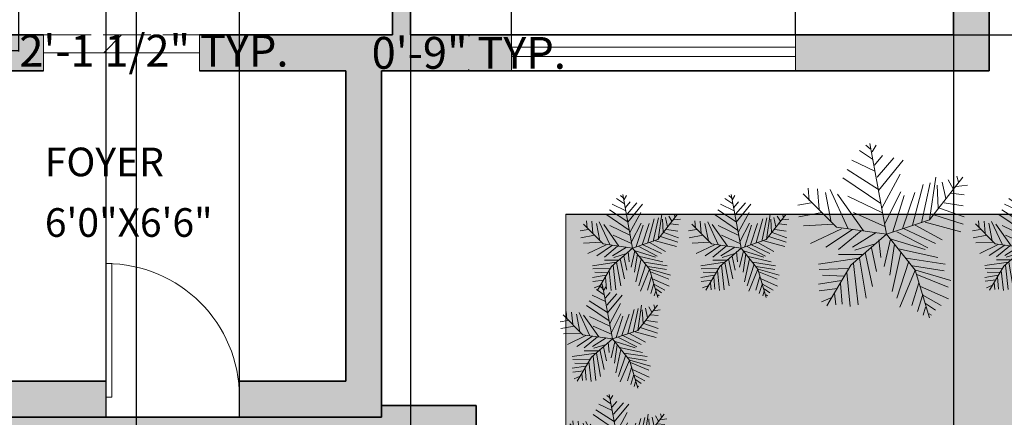
# Model space of a CAD drawing. Units: inches. Extents: x 853 to 1550, y 485 to 1596.
# Tile 5 of 18: x 1170 to 1418, y 768 to 867. Entities that reach past the tile are written whole.
import ezdxf

# ---------------------------------------------------------------- set-up
doc = ezdxf.new("R2010")
doc.units = ezdxf.units.IN
doc.header["$MEASUREMENT"] = 0
doc.linetypes.add('ACAD_ISO02W100', pattern=[15, 12, -3])
for name, color, linetype, lineweight in [('A-ANNO-DIMS', 2, 'Continuous', 18), ('A-AREA-IDEN', 250, 'Continuous', 18), ('A-DOOR', 4, 'Continuous', 18), ('A-GLAZ-HIDN', 4, 'ACAD_ISO02W100', 13), ('A-WALL-PATT', 250, 'Continuous', 13), ('L-PLNT-TREE', 106, 'Continuous', 13), ('lawn', 106, 'Continuous', 18), ('walls', 250, 'Continuous', 35), ('windows', 4, 'Continuous', 18)]:
    doc.layers.add(name, color=color, linetype=linetype, lineweight=lineweight)
doc.layers.add('A-FLOR-PATT', color=254, linetype='Continuous', lineweight=13, true_color=0xfeeab9)
doc.layers.add('L-PLNT-PATT', color=85, linetype='Continuous', lineweight=13, true_color=0x58ba48)
doc.styles.get("Standard").update_dxf_attribs({"font": 'arial.ttf'})
doc.dimstyles.get("Standard").update_dxf_attribs({"dimtxt": 8, "dimasz": 0.18, "dimexe": 0.18, "dimexo": 0.0625, "dimgap": 0.09, "dimtad": 0, "dimtih": 1, "dimtoh": 1, "dimzin": 0, "dimdsep": 46, "dimlunit": 3, "dimtxsty": 'Standard', "dimcen": 0.09, "dimadec": 0, "dimazin": 0, "dimtfac": 1, "dimtofl": 0, "dimtmove": 0, "dimatfit": 3, "dimfxl": 1, "dimtolj": 1, "dimtzin": 0, "dimarcsym": 0})

# ---------------------------------------------------------------- blocks, each defined once
blk = doc.blocks.new('*U10')
for p, q in [((0, 0), (0, -6)), ((40, 0), (40, -6))]:
    blk.add_line(p, q)
blk.add_lwpolyline([(0, 0), (0, 40), (1.75, 40), (1.75, 0)], close=True)
blk.add_arc((0, 0), 40, 0, 90)
blk = doc.blocks.new('*U18')
for p, q in [((-10.186, 53.64), (-13.084, 55.962)), ((0, 0), (-10.5, 57)), ((-9.099, 51.782), (-6.563, 55.962)), ((-8.737, 47.138), (-17.069, 52.711)), ((-7.288, 39.707), (-21.778, 46.673)), ((-7.65, 43.423), (-2.578, 49.46)), ((-5.839, 35.992), (4.667, 48.067)), ((-5.114, 27.632), (10.463, 46.673)), ((-5.114, 28.097), (-24.676, 40.636)), ((-2.941, 16.486), (8.652, 37.85)), ((-3.665, 19.273), (-27.574, 35.527)), ((16.259, 5.805), (23.142, 31.348)), ((22.055, 7.198), (27.489, 32.277)), ((27, 9), (48, 36)), ((27.127, 9.056), (31.112, 35.992)), ((35.096, 32.741), (37.27, 22.524)), ((38.719, 34.134), (41.979, 28.561)), ((44.153, 36.456), (45.239, 32.741)), ((-31.5, 4.5), (-52.5, 25.5)), ((-48.585, 21.131), (-49.309, 29.026)), ((-43.513, 28.561), (-42.427, 15.558)), ((-38.442, 26.239), (-34.819, 7.663)), ((-35.544, 28.097), (-24.314, 3.947)), ((-14.533, 2.09), (-30.834, 25.31)), ((-1.129, 6.734), (9.014, 26.704)), ((10.101, 3.483), (17.708, 26.239)), ((31.836, 30.883), (32.561, 16.486)), ((40.53, 25.775), (48.862, 24.846)), ((43.791, 29.954), (51.036, 30.883)), ((-47.498, 19.737), (-55.83, 18.344)), ((-24.314, 23.917), (-2.941, 13.7)), ((3.942, 1.625), (11.187, 24.381)), ((36.183, 19.737), (48.137, 17.88)), ((-40.615, 13.7), (-55.105, 10.913)), ((-20.691, 13.7), (-1.129, 4.876)), ((33.285, 16.486), (48.862, 10.913)), ((-33.37, 6.269), (-52.207, 5.34)), ((0, 0), (27, 9)), ((24.229, 7.663), (46.688, 1.625)), ((29.662, 12.307), (48.137, 6.269)), ((-28.299, 3.483), (-47.86, -5.805)), ((-21.416, 3.018), (-38.079, -8.128)), ((0, 0), (-31.5, 4.5)), ((-15.982, 2.09), (-30.11, -9.521)), ((0, 0), (-22.5, -19.5)), ((-6.563, 1.161), (-21.416, -8.128)), ((0, 0), (18, -22.5)), ((6.478, 1.625), (26.04, -8.592)), ((11.187, 3.483), (30.749, -5.805)), ((18.07, 5.805), (35.096, -3.483)), ((-6.563, -5.805), (-19.967, -9.985)), ((-4.752, -3.483), (-3.665, -14.629)), ((2.493, -3.019), (-1.491, -20.202)), ((1.769, -2.555), (24.229, -9.521)), ((-13.446, -11.378), (-8.737, -32.741)), ((-9.461, -8.592), (-6.201, -23.453)), ((5.029, -6.27), (2.131, -25.775)), ((9.014, -11.378), (3.58, -35.992)), ((7.565, -9.056), (32.198, -14.629)), ((-17.431, -15.094), (-42.789, -18.809)), ((-15.257, -12.772), (-30.11, -12.772)), ((-20.691, -18.345), (-17.793, -44.352)), ((-17.069, -15.094), (-12.721, -40.172)), ((14.085, -16.951), (6.478, -40.172)), ((12.274, -15.094), (36.907, -18.809)), ((-24.314, -21.596), (-42.427, -22.06)), ((-22.5, -19.5), (-37.5, -45)), ((-25.038, -23.918), (-22.865, -45.281)), ((18.07, -22.524), (8.289, -45.745)), ((16.259, -19.738), (36.183, -22.989)), ((18, -22.5), (27, -52.5)), ((18.433, -22.524), (40.53, -29.026)), ((-28.299, -29.026), (-42.789, -31.348)), ((-26.849, -26.24), (-40.253, -25.775)), ((-29.023, -30.884), (-27.936, -43.887)), ((20.244, -30.419), (15.897, -44.816)), ((19.157, -25.311), (38.719, -33.206)), ((-30.834, -34.135), (-42.427, -35.528)), ((-32.646, -36.921), (-31.921, -44.352)), ((21.331, -32.741), (39.081, -40.636)), ((-34.457, -39.708), (-40.978, -42.494)), ((22.78, -37.85), (19.519, -48.532)), ((22.78, -38.314), (34.372, -44.816)), ((24.591, -45.745), (23.142, -50.854)), ((24.591, -43.423), (30.749, -47.603)), ((26.764, -49.925), (28.213, -50.854))]:
    blk.add_line(p, q)
blk = doc.blocks.new('WIN-71IN')
for p, q in [((0, 9), (0, 0)), ((71.43, 9), (0, 9)), ((0, 9), (0, 5.92)), ((71.43, 0), (71.43, 9)), ((0, 5.92), (71.43, 5.92)), ((71.43, 5.92), (71.43, 3.59)), ((71.43, 3.59), (0, 3.59)), ((0, 0), (71.43, 0))]:
    blk.add_line(p, q)
blk = doc.blocks.new('*D41')
at = {"layer": 'A-ANNO-DIMS', "color": 0, "lineweight": -2, "transparency": 16777216}
for p, q in [((1293.81, 863.69), (1293.81, 874.52)), ((1293.99, 874.34), (1365.06, 874.34)), ((1365.24, 863.69), (1365.24, 874.52)), ((1365.24, 874.34), (1365.42, 874.34))]:
    blk.add_line(p, q, dxfattribs=at)
at = {"layer": 'A-ANNO-DIMS', "color": 0, "transparency": 16777216}
for points in [[(1293.99, 874.37), (1293.99, 874.31), (1293.81, 874.34)], [(1365.06, 874.37), (1365.06, 874.31), (1365.24, 874.34)]]:
    blk.add_solid(points, dxfattribs=at)
at = {"layer": 'Defpoints', "color": 0, "transparency": 16777216}
for p in [(1365.24, 874.34), (1293.81, 863.63), (1365.24, 863.63)]:
    blk.add_point(p, dxfattribs=at)
at = {"layer": 'A-ANNO-DIMS', "color": 0, "transparency": 16777216, "insert": (1428.56, 874.34), "char_height": 8, "attachment_point": 5}
blk.add_mtext('\\A1;WINDOW 5\'-11 1/2" TYP.', dxfattribs=at)
blk = doc.blocks.new('*D42')
at = {"layer": 'A-ANNO-DIMS', "color": 0, "lineweight": -2, "transparency": 16777216}
for p, q in [((1293.75, 863.63), (1282.92, 863.63)), ((1283.1, 863.45), (1283.1, 863.3)), ((1293.75, 854.63), (1282.92, 854.63)), ((1283.1, 854.81), (1283.1, 854.95))]:
    blk.add_line(p, q, dxfattribs=at)
at = {"layer": 'A-ANNO-DIMS', "color": 0, "transparency": 16777216}
for points in [[(1283.07, 863.45), (1283.13, 863.45), (1283.1, 863.63)], [(1283.07, 854.81), (1283.13, 854.81), (1283.1, 854.63)]]:
    blk.add_solid(points, dxfattribs=at)
at = {"layer": 'Defpoints', "color": 0, "transparency": 16777216}
for p in [(1283.1, 863.63), (1293.81, 863.63), (1293.81, 854.63)]:
    blk.add_point(p, dxfattribs=at)
at = {"layer": 'A-ANNO-DIMS', "color": 0, "transparency": 16777216, "insert": (1283.1, 859.13), "char_height": 8, "attachment_point": 5}
blk.add_mtext('\\A1;0\'-9" TYP.', dxfattribs=at)
blk = doc.blocks.new('*D50')
at = {"layer": 'A-ANNO-DIMS', "color": 0, "lineweight": -2, "transparency": 16777216}
for p, q in [((1144.37, 871.78), (1144.37, 859.5)), ((1169.9, 871.78), (1169.9, 859.5)), ((1144.55, 859.68), (1169.72, 859.68)), ((1169.9, 859.68), (1170.08, 859.68))]:
    blk.add_line(p, q, dxfattribs=at)
at = {"layer": 'A-ANNO-DIMS', "color": 0, "transparency": 16777216}
for points in [[(1144.55, 859.71), (1144.55, 859.65), (1144.37, 859.68)], [(1169.72, 859.71), (1169.72, 859.65), (1169.9, 859.68)]]:
    blk.add_solid(points, dxfattribs=at)
at = {"layer": 'Defpoints', "color": 0, "transparency": 16777216}
for p in [(1144.37, 871.84), (1169.9, 871.84), (1169.9, 859.68)]:
    blk.add_point(p, dxfattribs=at)
at = {"layer": 'A-ANNO-DIMS', "color": 0, "transparency": 16777216, "insert": (1203.94, 859.68), "char_height": 8, "attachment_point": 5}
blk.add_mtext('\\A1;2\'-1 1/2" TYP.', dxfattribs=at)
blk = doc.blocks.new('*D72')
at = {"layer": 'A-ANNO-DIMS', "color": 0, "lineweight": -2, "transparency": 16777216}
for p, q in [((1139.44, 1321.07), (1139.44, 497.1)), ((1199.44, 1321.07), (1199.44, 497.1)), ((1139.62, 497.28), (1158.71, 497.28)), ((1199.26, 497.28), (1180.16, 497.28))]:
    blk.add_line(p, q, dxfattribs=at)
at = {"layer": 'A-ANNO-DIMS', "color": 0, "transparency": 16777216}
for points in [[(1139.62, 497.31), (1139.62, 497.25), (1139.44, 497.28)], [(1199.26, 497.31), (1199.26, 497.25), (1199.44, 497.28)]]:
    blk.add_solid(points, dxfattribs=at)
at = {"layer": 'Defpoints', "color": 0, "transparency": 16777216}
for p in [(1139.44, 1321.13), (1199.44, 1321.13), (1199.44, 497.28)]:
    blk.add_point(p, dxfattribs=at)
at = {"layer": 'A-ANNO-DIMS', "color": 0, "transparency": 16777216, "insert": (1169.44, 497.28), "char_height": 8, "attachment_point": 5}
blk.add_mtext('\\A1;5\'-0"', dxfattribs=at)
blk = doc.blocks.new('*D74')
at = {"layer": 'A-ANNO-DIMS', "color": 0, "lineweight": -2, "transparency": 16777216}
for p, q in [((1268.44, 863.57), (1268.44, 497.1)), ((1404.94, 863.57), (1404.94, 497.1)), ((1268.62, 497.28), (1313.91, 497.28)), ((1404.76, 497.28), (1359.46, 497.28))]:
    blk.add_line(p, q, dxfattribs=at)
at = {"layer": 'A-ANNO-DIMS', "color": 0, "transparency": 16777216}
for points in [[(1268.62, 497.31), (1268.62, 497.25), (1268.44, 497.28)], [(1404.76, 497.31), (1404.76, 497.25), (1404.94, 497.28)]]:
    blk.add_solid(points, dxfattribs=at)
at = {"layer": 'Defpoints', "color": 0, "transparency": 16777216}
for p in [(1268.44, 863.63), (1404.94, 863.63), (1404.94, 497.28)]:
    blk.add_point(p, dxfattribs=at)
at = {"layer": 'A-ANNO-DIMS', "color": 0, "transparency": 16777216, "insert": (1336.69, 497.28), "char_height": 8, "attachment_point": 5}
blk.add_mtext('\\A1;11\'-4 1/2"', dxfattribs=at)
blk = doc.blocks.new('*D75')
at = {"layer": 'A-ANNO-DIMS', "color": 0, "lineweight": -2, "transparency": 16777216}
for p, q in [((1405, 1031.63), (1526.24, 1031.63)), ((1526.06, 1031.45), (1526.06, 951.8)), ((1526.06, 863.81), (1526.06, 943.45)), ((1405, 863.63), (1526.24, 863.63))]:
    blk.add_line(p, q, dxfattribs=at)
at = {"layer": 'A-ANNO-DIMS', "color": 0, "transparency": 16777216}
for points in [[(1526.03, 1031.45), (1526.09, 1031.45), (1526.06, 1031.63)], [(1526.03, 863.81), (1526.09, 863.81), (1526.06, 863.63)]]:
    blk.add_solid(points, dxfattribs=at)
at = {"layer": 'Defpoints', "color": 0, "transparency": 16777216}
for p in [(1404.94, 1031.63), (1526.06, 1031.63), (1404.94, 863.63)]:
    blk.add_point(p, dxfattribs=at)
at = {"layer": 'A-ANNO-DIMS', "color": 0, "transparency": 16777216, "insert": (1526.06, 947.63), "char_height": 8, "attachment_point": 5}
blk.add_mtext('\\A1;14\'-0"', dxfattribs=at)
blk = doc.blocks.new('*D80')
at = {"layer": 'A-ANNO-DIMS', "color": 0, "lineweight": -2, "transparency": 16777216}
for p, q in [((1307.55, 818.63), (1526.24, 818.63)), ((1526.06, 818.45), (1526.06, 755.21)), ((1526.06, 683.5), (1526.06, 746.75)), ((1307.55, 683.32), (1526.24, 683.32))]:
    blk.add_line(p, q, dxfattribs=at)
at = {"layer": 'A-ANNO-DIMS', "color": 0, "transparency": 16777216}
for points in [[(1526.03, 818.45), (1526.09, 818.45), (1526.06, 818.63)], [(1526.03, 683.5), (1526.09, 683.5), (1526.06, 683.32)]]:
    blk.add_solid(points, dxfattribs=at)
at = {"layer": 'Defpoints', "color": 0, "transparency": 16777216}
for p in [(1307.49, 818.63), (1526.06, 818.63), (1307.49, 683.32)]:
    blk.add_point(p, dxfattribs=at)
at = {"layer": 'A-ANNO-DIMS', "color": 0, "transparency": 16777216, "insert": (1526.06, 750.98), "char_height": 8, "attachment_point": 5}
blk.add_mtext('\\A1;11\'-3 1/2"', dxfattribs=at)
blk = doc.blocks.new('*D81')
at = {"layer": 'A-ANNO-DIMS', "color": 0, "lineweight": -2, "transparency": 16777216}
for p, q in [((1191.94, 767.69), (1191.94, 1584.65)), ((1192.12, 1584.47), (1225.27, 1584.47)), ((1225.45, 767.69), (1225.45, 1584.65)), ((1225.45, 1584.47), (1225.63, 1584.47))]:
    blk.add_line(p, q, dxfattribs=at)
at = {"layer": 'A-ANNO-DIMS', "color": 0, "transparency": 16777216}
for points in [[(1192.12, 1584.5), (1192.12, 1584.44), (1191.94, 1584.47)], [(1225.27, 1584.5), (1225.27, 1584.44), (1225.45, 1584.47)]]:
    blk.add_solid(points, dxfattribs=at)
at = {"layer": 'Defpoints', "color": 0, "transparency": 16777216}
for p in [(1225.45, 1584.47), (1191.94, 767.63), (1225.45, 767.63)]:
    blk.add_point(p, dxfattribs=at)
at = {"layer": 'A-ANNO-DIMS', "color": 0, "transparency": 16777216, "insert": (1245.74, 1584.47), "char_height": 8, "attachment_point": 5}
blk.add_mtext('\\A1;2\'-9 1/2"', dxfattribs=at)

msp = doc.modelspace()

# ---------------------------------------------------------------- hatches: boundary and pattern name
at = {"layer": 'A-FLOR-PATT'}
h = msp.add_hatch(color=256, dxfattribs=at)
h.dxf.hatch_style = 1
h.paths.add_polyline_path([(1113.94, 788.629), (1110.94, 788.629), (1110.94, 769.463), (1113.94, 769.463)])
h.paths.add_polyline_path([(1113.94, 768.501), (1110.94, 768.501), (1110.94, 707.356), (1113.94, 707.356)])
h.paths.add_polyline_path([(1276.896, 702.868), (1118.963, 702.868), (1118.963, 699.868), (1276.896, 699.868)])
h.paths.add_polyline_path([(1284.919, 770.496), (1261.179, 770.496), (1261.179, 767.496), (1281.919, 767.496), (1281.919, 707.356), (1284.919, 707.356)])
h = msp.add_hatch(color=256, dxfattribs=at)
h.dxf.hatch_style = 1
h.paths.add_polyline_path([(1281.919, 767.496), (1261.179, 767.496), (1113.94, 767.629), (1113.94, 707.356), (1118.963, 707.356), (1118.963, 702.868), (1276.896, 702.868), (1276.896, 707.356), (1281.919, 707.356)])
at = {"layer": 'A-WALL-PATT'}
h = msp.add_hatch(color=256, dxfattribs=at)
h.dxf.hatch_style = 1
h.paths.add_polyline_path([(1139.437, 988.732), (1134.937, 988.732), (1134.937, 830.473), (1139.437, 830.473)])
h.paths.add_polyline_path([(1413.937, 1052.227), (1404.937, 1052.227), (1404.937, 1036.129), (1308.937, 1036.129), (1308.937, 1045.033), (1304.437, 1045.033), (1304.437, 1030.033), (1308.937, 1030.033), (1308.937, 1031.629), (1404.937, 1031.629), (1404.937, 863.629), (1365.241, 863.629), (1365.241, 854.629), (1413.937, 854.629)])
h.paths.add_polyline_path([(1413.937, 1133.918), (1404.937, 1133.918), (1404.937, 1100.629), (1304.437, 1100.629), (1304.437, 1078.26), (1308.937, 1078.26), (1308.937, 1096.129), (1404.937, 1096.129), (1404.937, 1084.233), (1407.946, 1084.233), (1413.937, 1084.233)])
h.paths.add_polyline_path([(1268.437, 1417.129), (1288.974, 1417.129), (1288.974, 1426.129), (1244.597, 1426.129), (1244.597, 1417.129), (1263.937, 1417.129), (1263.937, 1321.129), (1260.34, 1321.129), (1260.34, 1316.629), (1263.937, 1316.629), (1263.937, 1283.505), (1268.437, 1283.505)])
h.paths.add_polyline_path([(1413.937, 1426.129), (1360.402, 1426.129), (1360.402, 1417.129), (1404.937, 1417.129), (1404.937, 1249.129), (1268.437, 1249.129), (1268.437, 1254.041), (1268.357, 1254.041), (1263.937, 1254.041), (1263.937, 1244.629), (1404.937, 1244.629), (1404.937, 1228.163), (1413.937, 1228.163)])
h.paths.add_polyline_path([(1215.842, 1426.129), (1184.201, 1426.129), (1184.201, 1417.129), (1199.437, 1417.129), (1199.437, 1321.129), (1172.101, 1321.129), (1172.101, 1316.629), (1229.433, 1316.629), (1229.433, 1321.129), (1203.937, 1321.129), (1203.937, 1417.129), (1215.842, 1417.129)])
h.paths.add_polyline_path([(1139.437, 1417.129), (1155.446, 1417.129), (1155.446, 1426.129), (1091.831, 1426.129), (1091.831, 1417.129), (1134.937, 1417.129), (1134.937, 1289.22), (1139.437, 1289.22), (1139.437, 1316.629), (1143.553, 1316.629), (1143.553, 1321.129), (1139.437, 1321.129)])
h.paths.add_polyline_path([(1139.437, 1255.161), (1134.937, 1255.161), (1134.937, 1249.129), (990.937, 1249.129), (990.937, 1417.129), (1020.402, 1417.129), (1020.402, 1426.129), (981.937, 1426.129), (981.937, 1205.535), (984.477, 1205.535), (990.937, 1205.535), (990.937, 1244.629), (1134.937, 1244.629), (1134.937, 1237.775), (1139.437, 1237.775)])
h = msp.add_hatch(color=256, dxfattribs=at)
h.dxf.hatch_style = 1
h.paths.add_polyline_path([(990.937, 1111.29), (981.937, 1111.29), (981.937, 1044.136), (984.946, 1044.136), (990.937, 1044.136), (990.937, 1072.129), (1045.609, 1072.129, -0.0272078), (1045.453, 1074.983), (1045.453, 1076.629), (990.937, 1076.629)], flags=17)
h.paths.add_polyline_path([(1091.437, 1072.129), (1139.437, 1072.129), (1139.437, 1206.521), (1134.937, 1206.521), (1134.937, 1076.629), (1071.734, 1076.629), (1071.734, 1074.983), (1071.734, 1072.129), (1086.937, 1072.129), (1086.937, 1012.129), (990.937, 1012.129), (981.937, 1012.129), (981.937, 944.409), (990.937, 944.409), (990.937, 1007.629), (1091.437, 1007.629)])
h.paths.add_polyline_path([(990.937, 872.981), (981.937, 872.981), (981.937, 788.629), (990.937, 788.629)])
h.paths.add_polyline_path([(1014.605, 800.886), (990.937, 800.886), (990.937, 796.386), (1014.605, 796.386)])
h.paths.add_polyline_path([(1134.937, 793.129), (1090.727, 793.129), (1090.727, 788.629), (1134.937, 788.629)])
h.paths.add_polyline_path([(1139.437, 800.892), (1134.937, 800.892), (1134.937, 788.629), (1113.94, 788.629), (1113.94, 767.629), (1139.437, 767.629), (1191.938, 767.629), (1191.938, 772.657), (1191.938, 776.629), (1139.437, 776.629)])
h.paths.add_polyline_path([(1131.331, 781.621), (1131.331, 775.236), (1118.809, 775.236), (1118.809, 781.621)], flags=16)
h.paths.add_polyline_path([(1131.331, 781.621), (1118.809, 781.621), (1118.809, 775.236), (1131.331, 775.236)], flags=0)
h.paths.add_polyline_path([(1118.963, 707.356), (1110.94, 707.356), (1110.94, 699.868), (1118.963, 699.868)])
h.paths.add_polyline_path([(1284.919, 707.356), (1276.896, 707.356), (1276.896, 699.868), (1284.919, 699.868)])
h.paths.add_polyline_path([(1293.812, 863.629), (1268.437, 863.629), (1268.437, 984.936), (1308.937, 984.936), (1308.937, 996.627), (1304.437, 996.627), (1304.437, 989.436), (1263.937, 989.436), (1263.937, 863.629), (1215.364, 863.629), (1215.364, 854.629), (1252.179, 854.629), (1252.179, 776.629), (1225.216, 776.629, -0.0297134), (1225.453, 772.657), (1225.453, 767.629), (1261.179, 767.629), (1261.179, 854.629), (1293.812, 854.629)])
h.paths.add_polyline_path([(1176.151, 863.629), (1139.437, 863.629), (1139.437, 854.629), (1176.151, 854.629)])
h.paths.add_polyline_path([(1134.937, 863.629), (1109.834, 863.629), (1109.834, 859.129), (1134.937, 859.129)])
h.paths.add_polyline_path([(1148.879, 950.672), (1144.374, 950.672), (1144.374, 874.094), (1148.879, 874.094)])
h.paths.add_polyline_path([(1079.778, 863.629), (990.937, 863.629), (990.937, 859.129), (1079.778, 859.129)])
at = {"layer": 'L-PLNT-PATT'}
h = msp.add_hatch(color=256, dxfattribs=at)
h.dxf.hatch_style = 1
h.paths.add_polyline_path([(1083.746, 765.455), (957.937, 765.455), (957.937, 604.895), (1121.13, 604.895), (1121.13, 618.052), (1135.564, 618.052), (1135.564, 604.895), (1152.247, 604.895), (1152.247, 610.626), (1152.247, 683.324), (1083.746, 683.324)])
h.paths.add_polyline_path([(1437.937, 818.629), (1307.486, 818.629), (1307.486, 683.324), (1249.908, 683.324), (1249.908, 667.104), (1249.908, 604.895), (1266.059, 604.895), (1266.059, 618.052), (1280.493, 618.052), (1280.493, 604.895), (1437.937, 604.895)])

# ---------------------------------------------------------------- linework, layer by layer
at = {"layer": 'A-GLAZ-HIDN'}
msp.add_line((1176.151, 863.629), (1215.364, 863.629), dxfattribs=at)
at = {"layer": 'lawn'}
for p, q in [((1437.937, 818.629), (1307.486, 818.629)), ((1307.486, 818.629), (1307.486, 683.324)), ((1383.67, 818.629), (1437.937, 818.629))]:
    msp.add_line(p, q, dxfattribs=at)
at = {"layer": 'walls'}
for p, q in [((1413.937, 1426.129), (1413.937, 854.629)), ((1404.937, 1031.629), (1404.937, 863.629)), ((1263.937, 863.629), (1263.937, 989.436)), ((1268.437, 863.629), (1268.437, 984.936)), ((1139.437, 863.629), (1176.151, 863.629)), ((1215.364, 863.629), (1263.937, 863.629)), ((1268.437, 863.629), (1404.937, 863.629)), ((1139.437, 854.629), (1176.151, 854.629)), ((1215.364, 854.629), (1252.179, 854.629)), ((1252.179, 854.629), (1252.179, 776.629)), ((1261.179, 854.629), (1261.179, 767.629)), ((1261.179, 854.629), (1413.937, 854.629)), ((1139.437, 776.629), (1191.938, 776.629)), ((1225.216, 776.629), (1252.179, 776.629)), ((1225.216, 776.629), (1252.179, 776.629)), ((1261.179, 770.496), (1284.919, 770.496)), ((1284.919, 770.496), (1284.919, 699.868)), ((1113.94, 767.629), (1261.179, 767.629)), ((1215.364, 767.629), (1261.179, 767.629))]:
    msp.add_line(p, q, dxfattribs=at)
at = {"layer": 'windows'}
for p, q in [((1176.151, 863.629), (1176.151, 854.629)), ((1195.757, 863.629), (1191.328, 859.129)), ((1215.364, 863.629), (1208.489, 863.629)), ((1215.364, 863.629), (1215.364, 854.629)), ((1176.151, 859.129), (1215.364, 859.129))]:
    msp.add_line(p, q, dxfattribs=at)

# ---------------------------------------------------------------- block references
at = {"layer": 'A-DOOR', "xscale": 0.8378663751028531, "yscale": 0.8378663751028531, "zscale": 0.8378663751028531}
msp.add_blockref('*U10', (1191.938, 772.657), dxfattribs=at)
at = {"layer": 'L-PLNT-TREE'}
for p, xscale, yscale, zscale in [((1388.119, 813.54), 0.3996992985476591, 0.3996992985476591, 0.3996992985476591), ((1324.288, 810.075), 0.2357951711934384, 0.2357951711934384, 0.2357951711934384), ((1351.537, 810.075), 0.2357951711934384, 0.2357951711934384, 0.2357951711934384), ((1422.886, 810.116), 0.2357951711934384, 0.2357951711934384, 0.2357951711934384), ((1319.221, 787.258), 0.2357951711934384, 0.2357951711934384, 0.2357951711934384), ((1320.889, 759.87), 0.2357951711934384, 0.2357951711934384, 0.2357951711934384)]:
    msp.add_blockref('*U18', p, dxfattribs=dict(at, xscale=xscale, yscale=yscale, zscale=zscale))
at = {"layer": 'windows'}
msp.add_blockref('WIN-71IN', (1293.812, 854.629), dxfattribs=at)

# ---------------------------------------------------------------- texts
at = {"layer": 'A-AREA-IDEN'}
for s, p in [('FOYER', (1176.527, 828.124)), ('6\'0"X6\'6"', (1176.527, 812.905))]:
    msp.add_text(s, height=7.1944, dxfattribs=at).set_placement(p)

# ---------------------------------------------------------------- dimensions: what is measured, and where the dimension line sits
at = {"layer": 'A-ANNO-DIMS'}
for base, p1, p2, picture, middle in [((1225.453, 1584.468), (1191.938, 767.629), (1225.453, 767.629), '*D81', (1245.744, 1584.468)), ((1199.437, 497.279), (1139.437, 1321.129), (1199.437, 1321.129), '*D72', (1169.437, 497.279)), ((1404.937, 497.279), (1268.437, 863.629), (1404.937, 863.629), '*D74', (1336.687, 497.279))]:
    dim = msp.add_linear_dim(base=base, p1=p1, p2=p2, dimstyle='Standard', override={"dimdec": 1, "dimlfac": 1, "dimrnd": 0, "dimzin": 1, "dimdsep": 46, "dimlunit": 4, "dimfrac": 2}, dxfattribs=at)
    dim.commit()
    dim.dimension.update_dxf_attribs({"geometry": picture, "text_midpoint": middle})
for base, p1, p2, picture, middle in [((1526.064, 1031.629), (1404.937, 863.629), (1404.937, 1031.629), '*D75', (1526.064, 947.629)), ((1526.064, 818.629), (1307.486, 683.324), (1307.486, 818.629), '*D80', (1526.064, 750.977))]:
    dim = msp.add_linear_dim(base=base, p1=p1, p2=p2, angle=90, dimstyle='Standard', override={"dimdec": 1, "dimlfac": 1, "dimrnd": 0, "dimzin": 1, "dimdsep": 46, "dimlunit": 4, "dimfrac": 2}, dxfattribs=at)
    dim.commit()
    dim.dimension.update_dxf_attribs({"geometry": picture, "text_midpoint": middle})
for base, p1, p2, text, picture, middle in [((1365.241, 874.344), (1293.812, 863.629), (1365.241, 863.629), 'WINDOW <> TYP.', '*D41', (1428.556, 874.344)), ((1169.9, 859.68), (1144.374, 871.842), (1169.9, 871.842), '<> TYP.', '*D50', (1203.941, 859.68))]:
    dim = msp.add_linear_dim(base=base, p1=p1, p2=p2, text=text, dimstyle='Standard', override={"dimdec": 1, "dimlfac": 1, "dimrnd": 0, "dimzin": 1, "dimdsep": 46, "dimlunit": 4, "dimfrac": 2}, dxfattribs=at)
    dim.commit()
    dim.dimension.update_dxf_attribs({"geometry": picture, "text_midpoint": middle})
dim = msp.add_linear_dim(base=(1283.098, 863.629), p1=(1293.812, 854.629), p2=(1293.812, 863.629), angle=90, text='<> TYP.', dimstyle='Standard', override={"dimdec": 1, "dimlfac": 1, "dimrnd": 0, "dimzin": 1, "dimdsep": 46, "dimlunit": 4, "dimfrac": 2}, dxfattribs=at)
dim.commit()
dim.dimension.update_dxf_attribs({"geometry": '*D42', "text_midpoint": (1283.098, 859.129)})

doc.saveas('drawing.dxf')
